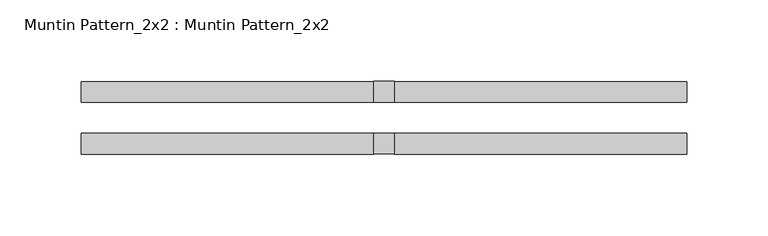
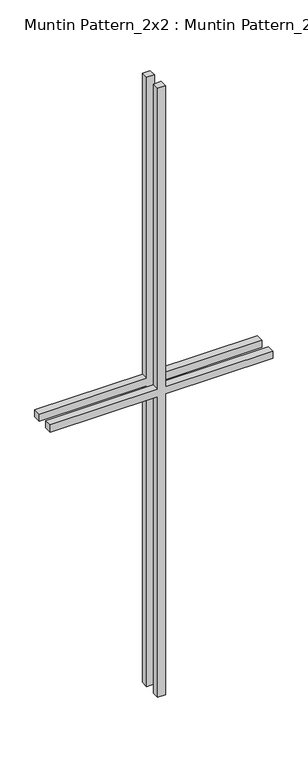
"""IFC4 building model written with IfcOpenShell, lengths in millimetres: proxy geometry, Muntin Pattern_2x2 : Muntin Pattern_2x2."""

from ifc_helpers import new_model, si_unit, frame, origin, place, context, project, spatial, polyline, outline, extrude, source, transform, mapped, element, save


def muntin_pattern_2x2_muntin_pattern_2x2_daa3f335(model_context):
    return source(origin(), model_context, "Body", "SweptSolid", [
        extrude(outline(polyline([(542.925, -6.35), (542.925, -185.7375), (530.225, -185.7375), (530.225, -6.35), (0.0, -6.35), (0.0, 6.35), (530.225, 6.35), (530.225, 185.7375), (542.925, 185.7375), (542.925, 6.35), (1073.15, 6.35), (1073.15, -6.35), (542.925, -6.35)])), frame((0.0, 9.525, 0.0), z_axis=(0.0, 1.0, 0.0), x_axis=(0.0, 0.0, 1.0)), (0.0, 0.0, 1.0), 12.7),
        extrude(outline(polyline([(542.925, -6.35), (542.925, -185.7375), (530.225, -185.7375), (530.225, -6.35), (0.0, -6.35), (0.0, 6.35), (530.225, 6.35), (530.225, 185.7375), (542.925, 185.7375), (542.925, 6.35), (1073.15, 6.35), (1073.15, -6.35), (542.925, -6.35)])), frame((0.0, -22.225, 0.0), z_axis=(0.0, 1.0, 0.0), x_axis=(0.0, 0.0, 1.0)), (0.0, 0.0, 1.0), 12.7),
    ])


if __name__ == "__main__":
    model = new_model("IFC4")
    model_context = context("Model", 3, world=origin())
    ifc_project = project(units=[si_unit("LENGTHUNIT", "METRE", prefix="MILLI")], contexts=[model_context])
    site = spatial("IfcSite", under=ifc_project)
    building = spatial("IfcBuilding", under=site)
    placement = place(None, origin())
    muntin_pattern_2x2_muntin_pattern_2x2_shape = muntin_pattern_2x2_muntin_pattern_2x2_daa3f335(model_context)
    element("IfcBuildingElementProxy", 1, Name="Muntin Pattern_2x2 : Muntin Pattern_2x2", ObjectType="Muntin Pattern_2x2 : Muntin Pattern_2x2", at=placement, inside=building, context=model_context, shape_type="MappedRepresentation", body=[
        mapped(muntin_pattern_2x2_muntin_pattern_2x2_shape, transform((0.0, 0.0, 0.0), x_axis=(1.0, 0.0, 0.0), y_axis=(0.0, 1.0, 0.0), z_axis=(0.0, 0.0, 1.0))),
    ])
    save(model, "model.ifc")

# Revit data of these elements
# Type "Muntin Pattern_2x2 : Muntin Pattern_2x2"
#   Width [instance default] = 4' - 0"
#   Thickness = 0' - 0 1/2"
#   Height [instance default] = 4' - 0"
#   Distance = 0' - 0 3/4"
#   Interior Material [instance default] = none
#   Exterior Material [instance default] = none
#   Default Elevation = 0
# Element 1 (IfcBuildingElementProxy, "Muntin Pattern_2x2 : Muntin Pattern_2x2")
#   Width = 1' - 2 5/8"
#   Height = 3' - 6 1/4"
#   Interior Material = Wood - Stained
#   Exterior Material = Clad - White
#   Materials on its faces: "Clad - White", "Wood - Stained"
# Materials
#   "Clad - White": class "Wood", colour RGB 242 242 238, transparency 0, Cost = 0
#   "Wood - Stained": class "Wood", colour RGB 224 178 126, transparency 0, Cost = 0
